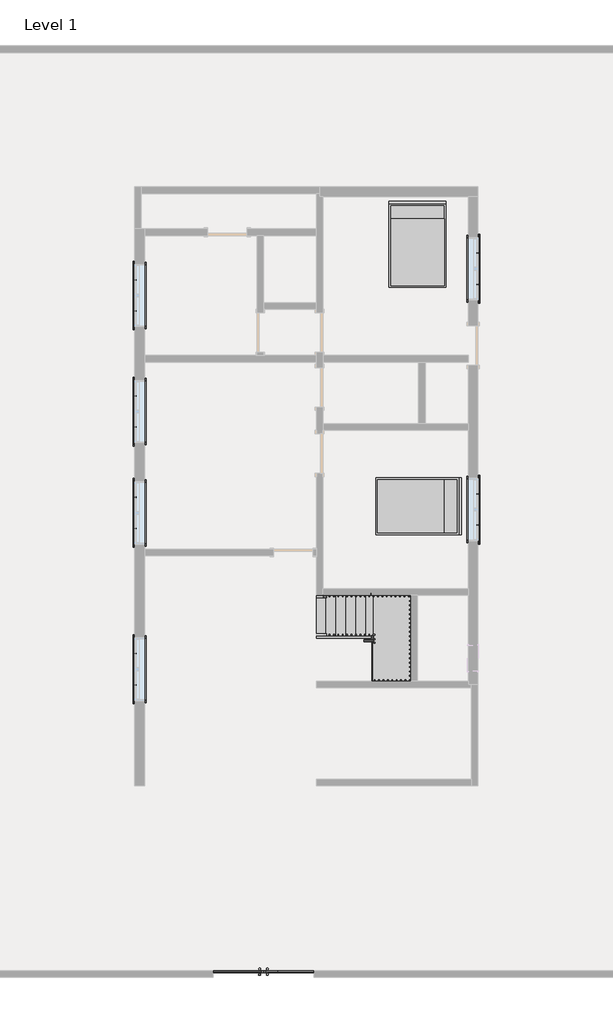
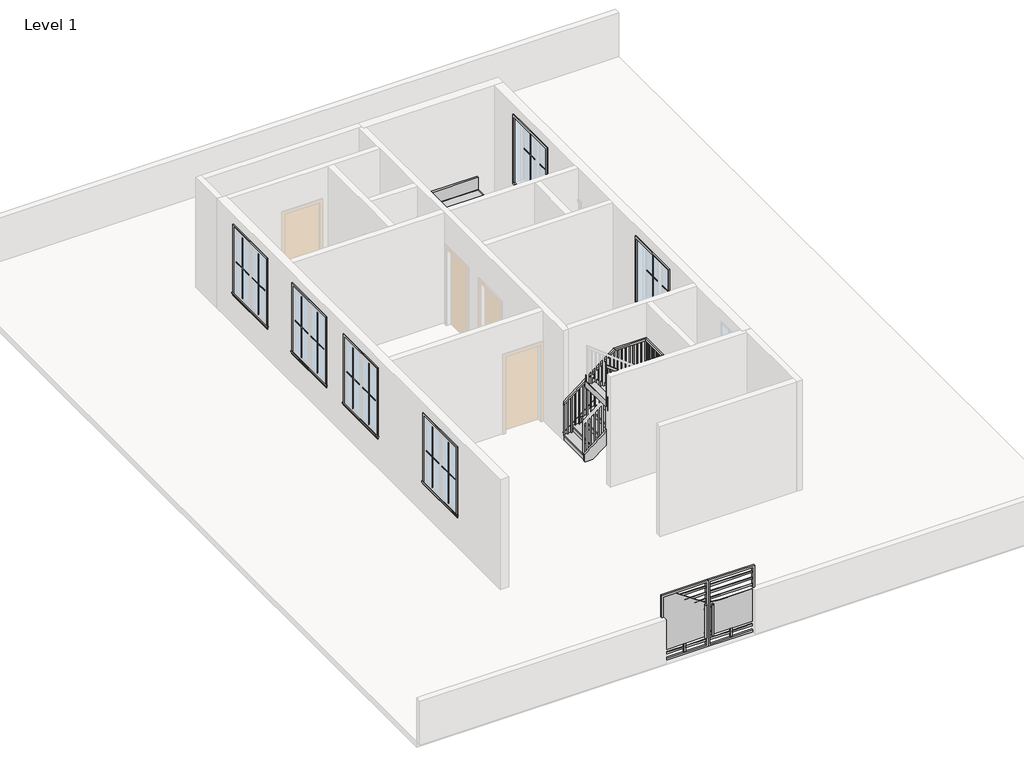
# One storey, part 2 of 2: 25 proxies, 6 members, 2 furniture elements, 1 railing, 1 stair flight.
"""IFC4 building model written with IfcOpenShell, lengths in millimetres."""

from ifc_helpers import new_model, si_unit, frame, origin, place, context, project, spatial, polyline, outline, extrude, faceted_brep, transform, mapped, element, save
from components import generic_models_113f6068, muntin_pattern_2x2_muntin_pattern_2x2_bff912c5, muntin_pattern_2x2_muntin_pattern_2x2_c2194282, trim_window_exterior_flat_with_sill_e04b3088, trim_window_interior_flat_picture_frame_2a7685fe, bed_17739_bed_17739_15c61121, stair_flight_3a0fea93

model = new_model("IFC4")

# Units and contexts
model_context = context("Model", 3, world=origin())
ifc_project = project(units=[si_unit("LENGTHUNIT", "METRE", prefix="MILLI")], contexts=[model_context])

# Site, building, storey
site = spatial("IfcSite", under=ifc_project)
building = spatial("IfcBuilding", under=site)
storey = spatial("IfcBuildingStorey", under=building, Name="Level 1", Elevation=0.0)

# Proxies
placement = place(None, origin())
generic_models_shape = generic_models_113f6068(model_context)
element("IfcBuildingElementProxy", 1, Name="Generic Models", at=placement, inside=storey, context=model_context, shape_type="MappedRepresentation", body=[
    mapped(generic_models_shape, transform((-2241.8415352, -11585.888028, 0.0), x_axis=(1.0, 0.0, 0.0), y_axis=(0.0, 1.0, 0.0), z_axis=(0.0, 0.0, 1.0))),
])
muntin_pattern_2x2_muntin_pattern_2x2_shape = muntin_pattern_2x2_muntin_pattern_2x2_bff912c5(model_context)
element("IfcBuildingElementProxy", 2, Name="Muntin Pattern_2x2 : Muntin Pattern_2x2", ObjectType="Muntin Pattern_2x2 : Muntin Pattern_2x2", at=placement, inside=storey, context=model_context, shape_type="MappedRepresentation", body=[
    mapped(muntin_pattern_2x2_muntin_pattern_2x2_shape, transform((-5204.1165352, 3633.8812696, 984.25), x_axis=(0.0, 1.0, 0.0), y_axis=(-1.0, 0.0, 0.0), z_axis=(0.0, 0.0, 1.0))),
])
element("IfcBuildingElementProxy", 3, Name="Muntin Pattern_2x2 : Muntin Pattern_2x2", ObjectType="Muntin Pattern_2x2 : Muntin Pattern_2x2", at=placement, inside=storey, context=model_context, shape_type="MappedRepresentation", body=[
    mapped(muntin_pattern_2x2_muntin_pattern_2x2_shape, transform((2701.6334648, 4971.3355313, 984.25), x_axis=(0.0, -1.0, 0.0), y_axis=(1.0, 0.0, 0.0), z_axis=(0.0, 0.0, 1.0))),
])
element("IfcBuildingElementProxy", 4, Name="Muntin Pattern_2x2 : Muntin Pattern_2x2", ObjectType="Muntin Pattern_2x2 : Muntin Pattern_2x2", at=placement, inside=storey, context=model_context, shape_type="MappedRepresentation", body=[
    mapped(muntin_pattern_2x2_muntin_pattern_2x2_shape, transform((2701.6334648, -584.9144687, 984.25), x_axis=(0.0, -1.0, 0.0), y_axis=(1.0, 0.0, 0.0), z_axis=(0.0, 0.0, 1.0))),
])
element("IfcBuildingElementProxy", 5, Name="Muntin Pattern_2x2 : Muntin Pattern_2x2", ObjectType="Muntin Pattern_2x2 : Muntin Pattern_2x2", at=placement, inside=storey, context=model_context, shape_type="MappedRepresentation", body=[
    mapped(muntin_pattern_2x2_muntin_pattern_2x2_shape, transform((-5204.1165352, 954.9605313, 984.25), x_axis=(0.0, 1.0, 0.0), y_axis=(-1.0, 0.0, 0.0), z_axis=(0.0, 0.0, 1.0))),
])
element("IfcBuildingElementProxy", 6, Name="Muntin Pattern_2x2 : Muntin Pattern_2x2", ObjectType="Muntin Pattern_2x2 : Muntin Pattern_2x2", at=placement, inside=storey, context=model_context, shape_type="MappedRepresentation", body=[
    mapped(muntin_pattern_2x2_muntin_pattern_2x2_shape, transform((-5204.1165352, -1381.8394687, 984.25), x_axis=(0.0, 1.0, 0.0), y_axis=(-1.0, 0.0, 0.0), z_axis=(0.0, 0.0, 1.0))),
])
element("IfcBuildingElementProxy", 7, Name="Muntin Pattern_2x2 : Muntin Pattern_2x2", ObjectType="Muntin Pattern_2x2 : Muntin Pattern_2x2", at=placement, inside=storey, context=model_context, shape_type="MappedRepresentation", body=[
    mapped(muntin_pattern_2x2_muntin_pattern_2x2_shape, transform((-5204.1165352, -4988.6394687, 984.25), x_axis=(0.0, 1.0, 0.0), y_axis=(-1.0, 0.0, 0.0), z_axis=(0.0, 0.0, 1.0))),
])
muntin_pattern_2x2_muntin_pattern_2x2_2_shape = muntin_pattern_2x2_muntin_pattern_2x2_c2194282(model_context)
element("IfcBuildingElementProxy", 8, Name="Muntin Pattern_2x2 : Muntin Pattern_2x2", ObjectType="Muntin Pattern_2x2 : Muntin Pattern_2x2", at=placement, inside=storey, context=model_context, shape_type="MappedRepresentation", body=[
    mapped(muntin_pattern_2x2_muntin_pattern_2x2_2_shape, transform((-5204.1165352, 4354.6062696, 984.25), x_axis=(0.0, -1.0, 0.0), y_axis=(1.0, 0.0, 0.0), z_axis=(0.0, 0.0, 1.0))),
])
element("IfcBuildingElementProxy", 9, Name="Muntin Pattern_2x2 : Muntin Pattern_2x2", ObjectType="Muntin Pattern_2x2 : Muntin Pattern_2x2", at=placement, inside=storey, context=model_context, shape_type="MappedRepresentation", body=[
    mapped(muntin_pattern_2x2_muntin_pattern_2x2_2_shape, transform((2701.6334648, 4250.6105313, 984.25), x_axis=(0.0, 1.0, 0.0), y_axis=(-1.0, 0.0, 0.0), z_axis=(0.0, 0.0, 1.0))),
])
element("IfcBuildingElementProxy", 10, Name="Muntin Pattern_2x2 : Muntin Pattern_2x2", ObjectType="Muntin Pattern_2x2 : Muntin Pattern_2x2", at=placement, inside=storey, context=model_context, shape_type="MappedRepresentation", body=[
    mapped(muntin_pattern_2x2_muntin_pattern_2x2_2_shape, transform((2701.6334648, -1305.6394687, 984.25), x_axis=(0.0, 1.0, 0.0), y_axis=(-1.0, 0.0, 0.0), z_axis=(0.0, 0.0, 1.0))),
])
element("IfcBuildingElementProxy", 11, Name="Muntin Pattern_2x2 : Muntin Pattern_2x2", ObjectType="Muntin Pattern_2x2 : Muntin Pattern_2x2", at=placement, inside=storey, context=model_context, shape_type="MappedRepresentation", body=[
    mapped(muntin_pattern_2x2_muntin_pattern_2x2_2_shape, transform((-5204.1165352, 1675.6855313, 984.25), x_axis=(0.0, -1.0, 0.0), y_axis=(1.0, 0.0, 0.0), z_axis=(0.0, 0.0, 1.0))),
])
element("IfcBuildingElementProxy", 12, Name="Muntin Pattern_2x2 : Muntin Pattern_2x2", ObjectType="Muntin Pattern_2x2 : Muntin Pattern_2x2", at=placement, inside=storey, context=model_context, shape_type="MappedRepresentation", body=[
    mapped(muntin_pattern_2x2_muntin_pattern_2x2_2_shape, transform((-5204.1165352, -661.1144687, 984.25), x_axis=(0.0, -1.0, 0.0), y_axis=(1.0, 0.0, 0.0), z_axis=(0.0, 0.0, 1.0))),
])
element("IfcBuildingElementProxy", 13, Name="Muntin Pattern_2x2 : Muntin Pattern_2x2", ObjectType="Muntin Pattern_2x2 : Muntin Pattern_2x2", at=placement, inside=storey, context=model_context, shape_type="MappedRepresentation", body=[
    mapped(muntin_pattern_2x2_muntin_pattern_2x2_2_shape, transform((-5204.1165352, -4267.9144687, 984.25), x_axis=(0.0, -1.0, 0.0), y_axis=(1.0, 0.0, 0.0), z_axis=(0.0, 0.0, 1.0))),
])
trim_window_exterior_flat_with_sill_shape = trim_window_exterior_flat_with_sill_e04b3088(model_context)
element("IfcBuildingElementProxy", 14, Name="Trim-Window-Exterior-Flat : with Sill", ObjectType="Trim-Window-Exterior-Flat : with Sill", at=placement, inside=storey, context=model_context, shape_type="MappedRepresentation", body=[
    mapped(trim_window_exterior_flat_with_sill_shape, transform((-5213.6415352, 3994.2437696, 2743.2), x_axis=(0.0, -1.0, 0.0), y_axis=(0.0, 0.0, 1.0), z_axis=(-1.0, 0.0, 0.0))),
])
element("IfcBuildingElementProxy", 15, Name="Trim-Window-Exterior-Flat : with Sill", ObjectType="Trim-Window-Exterior-Flat : with Sill", at=placement, inside=storey, context=model_context, shape_type="MappedRepresentation", body=[
    mapped(trim_window_exterior_flat_with_sill_shape, transform((2711.1584648, 4610.9730313, 2743.2), x_axis=(0.0, 1.0, 0.0), y_axis=(0.0, 0.0, 1.0), z_axis=(1.0, 0.0, 0.0))),
])
element("IfcBuildingElementProxy", 16, Name="Trim-Window-Exterior-Flat : with Sill", ObjectType="Trim-Window-Exterior-Flat : with Sill", at=placement, inside=storey, context=model_context, shape_type="MappedRepresentation", body=[
    mapped(trim_window_exterior_flat_with_sill_shape, transform((2711.1584648, -945.2769687, 2743.2), x_axis=(0.0, 1.0, 0.0), y_axis=(0.0, 0.0, 1.0), z_axis=(1.0, 0.0, 0.0))),
])
element("IfcBuildingElementProxy", 17, Name="Trim-Window-Exterior-Flat : with Sill", ObjectType="Trim-Window-Exterior-Flat : with Sill", at=placement, inside=storey, context=model_context, shape_type="MappedRepresentation", body=[
    mapped(trim_window_exterior_flat_with_sill_shape, transform((-5213.6415352, 1315.3230313, 2743.2), x_axis=(0.0, -1.0, 0.0), y_axis=(0.0, 0.0, 1.0), z_axis=(-1.0, 0.0, 0.0))),
])
element("IfcBuildingElementProxy", 18, Name="Trim-Window-Exterior-Flat : with Sill", ObjectType="Trim-Window-Exterior-Flat : with Sill", at=placement, inside=storey, context=model_context, shape_type="MappedRepresentation", body=[
    mapped(trim_window_exterior_flat_with_sill_shape, transform((-5213.6415352, -1021.4769687, 2743.2), x_axis=(0.0, -1.0, 0.0), y_axis=(0.0, 0.0, 1.0), z_axis=(-1.0, 0.0, 0.0))),
])
element("IfcBuildingElementProxy", 19, Name="Trim-Window-Exterior-Flat : with Sill", ObjectType="Trim-Window-Exterior-Flat : with Sill", at=placement, inside=storey, context=model_context, shape_type="MappedRepresentation", body=[
    mapped(trim_window_exterior_flat_with_sill_shape, transform((-5213.6415352, -4628.2769687, 2743.2), x_axis=(0.0, -1.0, 0.0), y_axis=(0.0, 0.0, 1.0), z_axis=(-1.0, 0.0, 0.0))),
])
trim_window_interior_flat_picture_frame_shape = trim_window_interior_flat_picture_frame_2a7685fe(model_context)
element("IfcBuildingElementProxy", 20, Name="Trim-Window-Interior-Flat : Picture Frame", ObjectType="Trim-Window-Interior-Flat : Picture Frame", at=placement, inside=storey, context=model_context, shape_type="MappedRepresentation", body=[
    mapped(trim_window_interior_flat_picture_frame_shape, transform((-4985.0415352, 3994.2437696, 2743.2), x_axis=(0.0, 1.0, 0.0), y_axis=(0.0, 0.0, 1.0), z_axis=(1.0, 0.0, 0.0))),
])
element("IfcBuildingElementProxy", 21, Name="Trim-Window-Interior-Flat : Picture Frame", ObjectType="Trim-Window-Interior-Flat : Picture Frame", at=placement, inside=storey, context=model_context, shape_type="MappedRepresentation", body=[
    mapped(trim_window_interior_flat_picture_frame_shape, transform((2482.5584648, 4610.9730313, 2743.2), x_axis=(0.0, -1.0, 0.0), y_axis=(0.0, 0.0, 1.0), z_axis=(-1.0, 0.0, 0.0))),
])
element("IfcBuildingElementProxy", 22, Name="Trim-Window-Interior-Flat : Picture Frame", ObjectType="Trim-Window-Interior-Flat : Picture Frame", at=placement, inside=storey, context=model_context, shape_type="MappedRepresentation", body=[
    mapped(trim_window_interior_flat_picture_frame_shape, transform((2482.5584648, -945.2769687, 2743.2), x_axis=(0.0, -1.0, 0.0), y_axis=(0.0, 0.0, 1.0), z_axis=(-1.0, 0.0, 0.0))),
])
element("IfcBuildingElementProxy", 23, Name="Trim-Window-Interior-Flat : Picture Frame", ObjectType="Trim-Window-Interior-Flat : Picture Frame", at=placement, inside=storey, context=model_context, shape_type="MappedRepresentation", body=[
    mapped(trim_window_interior_flat_picture_frame_shape, transform((-4985.0415352, 1315.3230313, 2743.2), x_axis=(0.0, 1.0, 0.0), y_axis=(0.0, 0.0, 1.0), z_axis=(1.0, 0.0, 0.0))),
])
element("IfcBuildingElementProxy", 24, Name="Trim-Window-Interior-Flat : Picture Frame", ObjectType="Trim-Window-Interior-Flat : Picture Frame", at=placement, inside=storey, context=model_context, shape_type="MappedRepresentation", body=[
    mapped(trim_window_interior_flat_picture_frame_shape, transform((-4985.0415352, -1021.4769687, 2743.2), x_axis=(0.0, 1.0, 0.0), y_axis=(0.0, 0.0, 1.0), z_axis=(1.0, 0.0, 0.0))),
])
element("IfcBuildingElementProxy", 25, Name="Trim-Window-Interior-Flat : Picture Frame", ObjectType="Trim-Window-Interior-Flat : Picture Frame", at=placement, inside=storey, context=model_context, shape_type="MappedRepresentation", body=[
    mapped(trim_window_interior_flat_picture_frame_shape, transform((-4985.0415352, -4628.2769687, 2743.2), x_axis=(0.0, 1.0, 0.0), y_axis=(0.0, 0.0, 1.0), z_axis=(1.0, 0.0, 0.0))),
])

# Furniture
bed_17739_bed_17739_shape = bed_17739_bed_17739_15c61121(model_context)
element("IfcFurniture", 26, ObjectType="Bed_17739 : Bed_17739", at=placement, inside=storey, context=model_context, shape_type="MappedRepresentation", body=[
    mapped(bed_17739_bed_17739_shape, transform((1314.1584648, 5149.1645078, 0.0), x_axis=(1.0, 0.0, 0.0), y_axis=(0.0, 1.0, 0.0), z_axis=(0.0, 0.0, 1.0))),
])
element("IfcFurniture", 27, ObjectType="Bed_17739 : Bed_17739", at=placement, inside=storey, context=model_context, shape_type="MappedRepresentation", body=[
    mapped(bed_17739_bed_17739_shape, transform((1314.1584648, -869.0769687, 0.0), x_axis=(0.0, -1.0, 0.0), y_axis=(1.0, 0.0, 0.0), z_axis=(0.0, 0.0, 1.0))),
])

# Members
element("IfcMember", 28, ObjectType="Stringer - 2\" Width", at=placement, inside=storey, context=model_context, shape_type="SweptSolid", body=[
    extrude(outline(polyline([(221.7399812, -1022.6415352), (0.0, -1022.6415352), (0.0, -811.2687863), (1261.5333333, 810.8400359), (1261.5333333, 314.3488758), (221.7399812, -1022.6415352)])), frame((0.0, -2926.4769687, 0.0), z_axis=(0.0, 1.0, 0.0), x_axis=(0.0, 0.0, 1.0)), (0.0, 0.0, 1.0), 50.8),
])
element("IfcMember", 29, ObjectType="Stringer - 2\" Width", at=placement, inside=storey, context=model_context, shape_type="SweptSolid", body=[
    extrude(outline(polyline([(1161.7584648, -2875.6769687), (1212.5584648, -2875.6769687), (1212.5584648, -4907.6769687), (1161.7584648, -4907.6769687), (1161.7584648, -2875.6769687)])), frame((0.0, 0.0, 956.7333333), z_axis=(0.0, 0.0, 1.0), x_axis=(1.0, 0.0, 0.0)), (0.0, 0.0, 1.0), 304.8),
])
element("IfcMember", 30, ObjectType="Stringer - 2\" Width", at=placement, inside=storey, context=model_context, shape_type="SweptSolid", body=[
    extrude(outline(polyline([(956.7333333, 884.5469698), (2439.9765283, -1022.6415352), (2053.8494451, -1022.6415352), (956.7333333, 388.0558097), (956.7333333, 884.5469698)])), frame((0.0, -4958.4769687, 0.0), z_axis=(0.0, 1.0, 0.0), x_axis=(0.0, 0.0, 1.0)), (0.0, 0.0, 1.0), 50.8),
])
element("IfcMember", 31, ObjectType="Stringer - 2\" Width", at=placement, inside=storey, context=model_context, shape_type="SweptSolid", body=[
    extrude(outline(polyline([(221.7399812, -1022.6415352), (0.0, -1022.6415352), (0.0, -811.2687863), (820.5567404, 243.8221038), (1206.6838236, 243.8221038), (221.7399812, -1022.6415352)])), frame((0.0, -3912.0539367, 0.0), z_axis=(0.0, 1.0, 0.0), x_axis=(0.0, 0.0, 1.0)), (0.0, 0.0, 1.0), 50.8),
])
element("IfcMember", 32, ObjectType="Stringer - 2\" Width", at=placement, inside=storey, context=model_context, shape_type="SweptSolid", body=[
    extrude(outline(polyline([(243.8221038, -3861.2539367), (294.6221038, -3861.2539367), (294.6221038, -3942.4769687), (243.8221038, -3942.4769687), (243.8221038, -3861.2539367)])), frame((0.0, 0.0, 956.7333333), z_axis=(0.0, 0.0, 1.0), x_axis=(1.0, 0.0, 0.0)), (0.0, 0.0, 1.0), 304.8),
])
element("IfcMember", 33, ObjectType="Stringer - 2\" Width", at=placement, inside=storey, context=model_context, shape_type="SweptSolid", body=[
    extrude(outline(polyline([(1029.3978382, 294.6221038), (1415.5249214, 294.6221038), (2439.9765283, -1022.6415352), (2053.8494451, -1022.6415352), (1029.3978382, 294.6221038)])), frame((0.0, -3993.2769687, 0.0), z_axis=(0.0, 1.0, 0.0), x_axis=(0.0, 0.0, 1.0)), (0.0, 0.0, 1.0), 50.8),
])

# Railing
element("IfcRailing", 34, ObjectType="Handrail - Rectangular", at=placement, inside=storey, context=model_context, shape_type="SolidModel", body=[
    faceted_brep([(-1022.6415352, -2926.4769687, 1083.7333333), (-1022.6415352, -2926.4769687, 1019.5783974), (-1022.6415352, -2977.2769687, 1019.5783974), (-1022.6415352, -2977.2769687, 1083.7333333), (294.6221038, -2926.4769687, 2099.7333333), (311.9370364, -2926.4769687, 2048.9333333), (311.9370364, -2977.2769687, 2048.9333333), (294.6221038, -2977.2769687, 2099.7333333), (1161.7584648, -2926.4769687, 2099.7333333), (1161.7584648, -2926.4769687, 2048.9333333), (1110.9584648, -2977.2769687, 2048.9333333), (1110.9584648, -2977.2769687, 2099.7333333), (1161.7584648, -4907.6769687, 2099.7333333), (1161.7584648, -4907.6769687, 2048.9333333), (1110.9584648, -4856.8769687, 2048.9333333), (1110.9584648, -4856.8769687, 2099.7333333), (514.1660437, -4907.6769687, 2099.7333333), (496.8511111, -4907.6769687, 2048.9333333), (496.8511111, -4856.8769687, 2048.9333333), (514.1660437, -4856.8769687, 2099.7333333), (-1022.6415352, -4907.6769687, 3285.0666667), (-1022.6415352, -4856.8769687, 3285.0666667), (-1022.6415352, -4856.8769687, 3220.9117307), (-1022.6415352, -4907.6769687, 3220.9117307)], [[[0, 1, 2, 3]], [[1, 0, 4, 5]], [[2, 1, 5, 6]], [[3, 2, 6, 7]], [[0, 3, 7, 4]], [[5, 4, 8, 9]], [[6, 5, 9, 10]], [[7, 6, 10, 11]], [[4, 7, 11, 8]], [[9, 8, 12, 13]], [[10, 9, 13, 14]], [[11, 10, 14, 15]], [[8, 11, 15, 12]], [[13, 12, 16, 17]], [[14, 13, 17, 18]], [[15, 14, 18, 19]], [[12, 15, 19, 16]], [[20, 21, 22, 23]], [[17, 16, 20, 23]], [[18, 17, 23, 22]], [[19, 18, 22, 21]], [[16, 19, 21, 20]]]),
    extrude(outline(polyline([(3208.6674089, -1006.7665352), (2201.3333333, -1006.7665352), (2201.3333333, -987.7165352), (3193.9742226, -987.7165352), (3208.6674089, -1006.7665352)])), frame((0.0, -4891.8019687, 0.0), z_axis=(0.0, 1.0, 0.0), x_axis=(0.0, 0.0, 1.0)), (0.0, 0.0, 1.0), 19.05),
    extrude(outline(polyline([(3130.3037488, -905.1665352), (2201.3333333, -905.1665352), (2201.3333333, -886.1165352), (3115.6105626, -886.1165352), (3130.3037488, -905.1665352)])), frame((0.0, -4891.8019687, 0.0), z_axis=(0.0, 1.0, 0.0), x_axis=(0.0, 0.0, 1.0)), (0.0, 0.0, 1.0), 19.05),
    extrude(outline(polyline([(3051.9400888, -803.5665352), (2201.3333333, -803.5665352), (2201.3333333, -784.5165352), (3037.2469025, -784.5165352), (3051.9400888, -803.5665352)])), frame((0.0, -4891.8019687, 0.0), z_axis=(0.0, 1.0, 0.0), x_axis=(0.0, 0.0, 1.0)), (0.0, 0.0, 1.0), 19.05),
    extrude(outline(polyline([(2973.5764287, -701.9665352), (2032.0, -701.9665352), (2032.0, -682.9165352), (2958.8832425, -682.9165352), (2973.5764287, -701.9665352)])), frame((0.0, -4891.8019687, 0.0), z_axis=(0.0, 1.0, 0.0), x_axis=(0.0, 0.0, 1.0)), (0.0, 0.0, 1.0), 19.05),
    extrude(outline(polyline([(2895.2127687, -600.3665352), (2032.0, -600.3665352), (2032.0, -581.3165352), (2880.5195824, -581.3165352), (2895.2127687, -600.3665352)])), frame((0.0, -4891.8019687, 0.0), z_axis=(0.0, 1.0, 0.0), x_axis=(0.0, 0.0, 1.0)), (0.0, 0.0, 1.0), 19.05),
    extrude(outline(polyline([(2816.8491086, -498.7665352), (1862.6666667, -498.7665352), (1862.6666667, -479.7165352), (2802.1559224, -479.7165352), (2816.8491086, -498.7665352)])), frame((0.0, -4891.8019687, 0.0), z_axis=(0.0, 1.0, 0.0), x_axis=(0.0, 0.0, 1.0)), (0.0, 0.0, 1.0), 19.05),
    extrude(outline(polyline([(2738.4854486, -397.1665352), (1862.6666667, -397.1665352), (1862.6666667, -378.1165352), (2723.7922623, -378.1165352), (2738.4854486, -397.1665352)])), frame((0.0, -4891.8019687, 0.0), z_axis=(0.0, 1.0, 0.0), x_axis=(0.0, 0.0, 1.0)), (0.0, 0.0, 1.0), 19.05),
    extrude(outline(polyline([(2660.1217885, -295.5665352), (1693.3333333, -295.5665352), (1693.3333333, -276.5165352), (2645.4286023, -276.5165352), (2660.1217885, -295.5665352)])), frame((0.0, -4891.8019687, 0.0), z_axis=(0.0, 1.0, 0.0), x_axis=(0.0, 0.0, 1.0)), (0.0, 0.0, 1.0), 19.05),
    extrude(outline(polyline([(2581.7581285, -193.9665352), (1693.3333333, -193.9665352), (1693.3333333, -174.9165352), (2567.0649422, -174.9165352), (2581.7581285, -193.9665352)])), frame((0.0, -4891.8019687, 0.0), z_axis=(0.0, 1.0, 0.0), x_axis=(0.0, 0.0, 1.0)), (0.0, 0.0, 1.0), 19.05),
    extrude(outline(polyline([(2503.3944684, -92.3665352), (1524.0, -92.3665352), (1524.0, -73.3165352), (2488.7012822, -73.3165352), (2503.3944684, -92.3665352)])), frame((0.0, -4891.8019687, 0.0), z_axis=(0.0, 1.0, 0.0), x_axis=(0.0, 0.0, 1.0)), (0.0, 0.0, 1.0), 19.05),
    extrude(outline(polyline([(2425.0308084, 9.2334648), (1524.0, 9.2334648), (1524.0, 28.2834648), (2410.3376221, 28.2834648), (2425.0308084, 9.2334648)])), frame((0.0, -4891.8019687, 0.0), z_axis=(0.0, 1.0, 0.0), x_axis=(0.0, 0.0, 1.0)), (0.0, 0.0, 1.0), 19.05),
    extrude(outline(polyline([(2346.6671484, 110.8334648), (1524.0, 110.8334648), (1524.0, 129.8834648), (2331.9739621, 129.8834648), (2346.6671484, 110.8334648)])), frame((0.0, -4891.8019687, 0.0), z_axis=(0.0, 1.0, 0.0), x_axis=(0.0, 0.0, 1.0)), (0.0, 0.0, 1.0), 19.05),
    extrude(outline(polyline([(2268.3034883, 212.4334648), (1354.6666667, 212.4334648), (1354.6666667, 231.4834648), (2253.6103021, 231.4834648), (2268.3034883, 212.4334648)])), frame((0.0, -4891.8019687, 0.0), z_axis=(0.0, 1.0, 0.0), x_axis=(0.0, 0.0, 1.0)), (0.0, 0.0, 1.0), 19.05),
    extrude(outline(polyline([(2189.9398283, 314.0334648), (1185.3333333, 314.0334648), (1185.3333333, 333.0834648), (2175.246642, 333.0834648), (2189.9398283, 314.0334648)])), frame((0.0, -4891.8019687, 0.0), z_axis=(0.0, 1.0, 0.0), x_axis=(0.0, 0.0, 1.0)), (0.0, 0.0, 1.0), 19.05),
    extrude(outline(polyline([(2111.5761682, 415.6334648), (1185.3333333, 415.6334648), (1185.3333333, 434.6834648), (2096.882982, 434.6834648), (2111.5761682, 415.6334648)])), frame((0.0, -4891.8019687, 0.0), z_axis=(0.0, 1.0, 0.0), x_axis=(0.0, 0.0, 1.0)), (0.0, 0.0, 1.0), 19.05),
    extrude(outline(polyline([(536.2834648, -4891.8019687), (517.2334648, -4891.8019687), (517.2334648, -4872.7519687), (536.2834648, -4872.7519687), (536.2834648, -4891.8019687)])), frame((0.0, 0.0, 1185.3333333), z_axis=(0.0, 0.0, 1.0), x_axis=(1.0, 0.0, 0.0)), (0.0, 0.0, 1.0), 863.6),
    extrude(outline(polyline([(637.8834648, -4891.8019687), (618.8334648, -4891.8019687), (618.8334648, -4872.7519687), (637.8834648, -4872.7519687), (637.8834648, -4891.8019687)])), frame((0.0, 0.0, 1185.3333333), z_axis=(0.0, 0.0, 1.0), x_axis=(1.0, 0.0, 0.0)), (0.0, 0.0, 1.0), 863.6),
    extrude(outline(polyline([(739.4834648, -4891.8019687), (720.4334648, -4891.8019687), (720.4334648, -4872.7519687), (739.4834648, -4872.7519687), (739.4834648, -4891.8019687)])), frame((0.0, 0.0, 1185.3333333), z_axis=(0.0, 0.0, 1.0), x_axis=(1.0, 0.0, 0.0)), (0.0, 0.0, 1.0), 863.6),
    extrude(outline(polyline([(841.0834648, -4891.8019687), (822.0334648, -4891.8019687), (822.0334648, -4872.7519687), (841.0834648, -4872.7519687), (841.0834648, -4891.8019687)])), frame((0.0, 0.0, 1185.3333333), z_axis=(0.0, 0.0, 1.0), x_axis=(1.0, 0.0, 0.0)), (0.0, 0.0, 1.0), 863.6),
    extrude(outline(polyline([(942.6834648, -4891.8019687), (923.6334648, -4891.8019687), (923.6334648, -4872.7519687), (942.6834648, -4872.7519687), (942.6834648, -4891.8019687)])), frame((0.0, 0.0, 1185.3333333), z_axis=(0.0, 0.0, 1.0), x_axis=(1.0, 0.0, 0.0)), (0.0, 0.0, 1.0), 863.6),
    extrude(outline(polyline([(1044.2834648, -4891.8019687), (1025.2334648, -4891.8019687), (1025.2334648, -4872.7519687), (1044.2834648, -4872.7519687), (1044.2834648, -4891.8019687)])), frame((0.0, 0.0, 1185.3333333), z_axis=(0.0, 0.0, 1.0), x_axis=(1.0, 0.0, 0.0)), (0.0, 0.0, 1.0), 863.6),
    extrude(outline(polyline([(1145.8834648, -4771.1519687), (1145.8834648, -4790.2019687), (1126.8334648, -4790.2019687), (1126.8334648, -4771.1519687), (1145.8834648, -4771.1519687)])), frame((0.0, 0.0, 1185.3333333), z_axis=(0.0, 0.0, 1.0), x_axis=(1.0, 0.0, 0.0)), (0.0, 0.0, 1.0), 863.6),
    extrude(outline(polyline([(1145.8834648, -4669.5519687), (1145.8834648, -4688.6019687), (1126.8334648, -4688.6019687), (1126.8334648, -4669.5519687), (1145.8834648, -4669.5519687)])), frame((0.0, 0.0, 1185.3333333), z_axis=(0.0, 0.0, 1.0), x_axis=(1.0, 0.0, 0.0)), (0.0, 0.0, 1.0), 863.6),
    extrude(outline(polyline([(1145.8834648, -4567.9519687), (1145.8834648, -4587.0019687), (1126.8334648, -4587.0019687), (1126.8334648, -4567.9519687), (1145.8834648, -4567.9519687)])), frame((0.0, 0.0, 1185.3333333), z_axis=(0.0, 0.0, 1.0), x_axis=(1.0, 0.0, 0.0)), (0.0, 0.0, 1.0), 863.6),
    extrude(outline(polyline([(1145.8834648, -4466.3519687), (1145.8834648, -4485.4019687), (1126.8334648, -4485.4019687), (1126.8334648, -4466.3519687), (1145.8834648, -4466.3519687)])), frame((0.0, 0.0, 1185.3333333), z_axis=(0.0, 0.0, 1.0), x_axis=(1.0, 0.0, 0.0)), (0.0, 0.0, 1.0), 863.6),
    extrude(outline(polyline([(1145.8834648, -4364.7519687), (1145.8834648, -4383.8019687), (1126.8334648, -4383.8019687), (1126.8334648, -4364.7519687), (1145.8834648, -4364.7519687)])), frame((0.0, 0.0, 1185.3333333), z_axis=(0.0, 0.0, 1.0), x_axis=(1.0, 0.0, 0.0)), (0.0, 0.0, 1.0), 863.6),
    extrude(outline(polyline([(1145.8834648, -4263.1519687), (1145.8834648, -4282.2019687), (1126.8334648, -4282.2019687), (1126.8334648, -4263.1519687), (1145.8834648, -4263.1519687)])), frame((0.0, 0.0, 1185.3333333), z_axis=(0.0, 0.0, 1.0), x_axis=(1.0, 0.0, 0.0)), (0.0, 0.0, 1.0), 863.6),
    extrude(outline(polyline([(1145.8834648, -4161.5519687), (1145.8834648, -4180.6019687), (1126.8334648, -4180.6019687), (1126.8334648, -4161.5519687), (1145.8834648, -4161.5519687)])), frame((0.0, 0.0, 1185.3333333), z_axis=(0.0, 0.0, 1.0), x_axis=(1.0, 0.0, 0.0)), (0.0, 0.0, 1.0), 863.6),
    extrude(outline(polyline([(1145.8834648, -4059.9519687), (1145.8834648, -4079.0019687), (1126.8334648, -4079.0019687), (1126.8334648, -4059.9519687), (1145.8834648, -4059.9519687)])), frame((0.0, 0.0, 1185.3333333), z_axis=(0.0, 0.0, 1.0), x_axis=(1.0, 0.0, 0.0)), (0.0, 0.0, 1.0), 863.6),
    extrude(outline(polyline([(1145.8834648, -3958.3519687), (1145.8834648, -3977.4019687), (1126.8334648, -3977.4019687), (1126.8334648, -3958.3519687), (1145.8834648, -3958.3519687)])), frame((0.0, 0.0, 1185.3333333), z_axis=(0.0, 0.0, 1.0), x_axis=(1.0, 0.0, 0.0)), (0.0, 0.0, 1.0), 863.6),
    extrude(outline(polyline([(1145.8834648, -3856.7519687), (1145.8834648, -3875.8019687), (1126.8334648, -3875.8019687), (1126.8334648, -3856.7519687), (1145.8834648, -3856.7519687)])), frame((0.0, 0.0, 1185.3333333), z_axis=(0.0, 0.0, 1.0), x_axis=(1.0, 0.0, 0.0)), (0.0, 0.0, 1.0), 863.6),
    extrude(outline(polyline([(1145.8834648, -3755.1519687), (1145.8834648, -3774.2019687), (1126.8334648, -3774.2019687), (1126.8334648, -3755.1519687), (1145.8834648, -3755.1519687)])), frame((0.0, 0.0, 1185.3333333), z_axis=(0.0, 0.0, 1.0), x_axis=(1.0, 0.0, 0.0)), (0.0, 0.0, 1.0), 863.6),
    extrude(outline(polyline([(1145.8834648, -3653.5519687), (1145.8834648, -3672.6019687), (1126.8334648, -3672.6019687), (1126.8334648, -3653.5519687), (1145.8834648, -3653.5519687)])), frame((0.0, 0.0, 1185.3333333), z_axis=(0.0, 0.0, 1.0), x_axis=(1.0, 0.0, 0.0)), (0.0, 0.0, 1.0), 863.6),
    extrude(outline(polyline([(1145.8834648, -3551.9519687), (1145.8834648, -3571.0019687), (1126.8334648, -3571.0019687), (1126.8334648, -3551.9519687), (1145.8834648, -3551.9519687)])), frame((0.0, 0.0, 1185.3333333), z_axis=(0.0, 0.0, 1.0), x_axis=(1.0, 0.0, 0.0)), (0.0, 0.0, 1.0), 863.6),
    extrude(outline(polyline([(1145.8834648, -3450.3519687), (1145.8834648, -3469.4019687), (1126.8334648, -3469.4019687), (1126.8334648, -3450.3519687), (1145.8834648, -3450.3519687)])), frame((0.0, 0.0, 1185.3333333), z_axis=(0.0, 0.0, 1.0), x_axis=(1.0, 0.0, 0.0)), (0.0, 0.0, 1.0), 863.6),
    extrude(outline(polyline([(1145.8834648, -3348.7519687), (1145.8834648, -3367.8019687), (1126.8334648, -3367.8019687), (1126.8334648, -3348.7519687), (1145.8834648, -3348.7519687)])), frame((0.0, 0.0, 1185.3333333), z_axis=(0.0, 0.0, 1.0), x_axis=(1.0, 0.0, 0.0)), (0.0, 0.0, 1.0), 863.6),
    extrude(outline(polyline([(1145.8834648, -3247.1519687), (1145.8834648, -3266.2019687), (1126.8334648, -3266.2019687), (1126.8334648, -3247.1519687), (1145.8834648, -3247.1519687)])), frame((0.0, 0.0, 1185.3333333), z_axis=(0.0, 0.0, 1.0), x_axis=(1.0, 0.0, 0.0)), (0.0, 0.0, 1.0), 863.6),
    extrude(outline(polyline([(1145.8834648, -3145.5519687), (1145.8834648, -3164.6019687), (1126.8334648, -3164.6019687), (1126.8334648, -3145.5519687), (1145.8834648, -3145.5519687)])), frame((0.0, 0.0, 1185.3333333), z_axis=(0.0, 0.0, 1.0), x_axis=(1.0, 0.0, 0.0)), (0.0, 0.0, 1.0), 863.6),
    extrude(outline(polyline([(1145.8834648, -3043.9519687), (1145.8834648, -3063.0019687), (1126.8334648, -3063.0019687), (1126.8334648, -3043.9519687), (1145.8834648, -3043.9519687)])), frame((0.0, 0.0, 1185.3333333), z_axis=(0.0, 0.0, 1.0), x_axis=(1.0, 0.0, 0.0)), (0.0, 0.0, 1.0), 863.6),
    extrude(outline(polyline([(1101.4334648, -2942.3519687), (1120.4834648, -2942.3519687), (1120.4834648, -2961.4019687), (1101.4334648, -2961.4019687), (1101.4334648, -2942.3519687)])), frame((0.0, 0.0, 1185.3333333), z_axis=(0.0, 0.0, 1.0), x_axis=(1.0, 0.0, 0.0)), (0.0, 0.0, 1.0), 863.6),
    extrude(outline(polyline([(999.8334648, -2942.3519687), (1018.8834648, -2942.3519687), (1018.8834648, -2961.4019687), (999.8334648, -2961.4019687), (999.8334648, -2942.3519687)])), frame((0.0, 0.0, 1185.3333333), z_axis=(0.0, 0.0, 1.0), x_axis=(1.0, 0.0, 0.0)), (0.0, 0.0, 1.0), 863.6),
    extrude(outline(polyline([(898.2334648, -2942.3519687), (917.2834648, -2942.3519687), (917.2834648, -2961.4019687), (898.2334648, -2961.4019687), (898.2334648, -2942.3519687)])), frame((0.0, 0.0, 1185.3333333), z_axis=(0.0, 0.0, 1.0), x_axis=(1.0, 0.0, 0.0)), (0.0, 0.0, 1.0), 863.6),
    extrude(outline(polyline([(796.6334648, -2942.3519687), (815.6834648, -2942.3519687), (815.6834648, -2961.4019687), (796.6334648, -2961.4019687), (796.6334648, -2942.3519687)])), frame((0.0, 0.0, 1185.3333333), z_axis=(0.0, 0.0, 1.0), x_axis=(1.0, 0.0, 0.0)), (0.0, 0.0, 1.0), 863.6),
    extrude(outline(polyline([(695.0334648, -2942.3519687), (714.0834648, -2942.3519687), (714.0834648, -2961.4019687), (695.0334648, -2961.4019687), (695.0334648, -2942.3519687)])), frame((0.0, 0.0, 1185.3333333), z_axis=(0.0, 0.0, 1.0), x_axis=(1.0, 0.0, 0.0)), (0.0, 0.0, 1.0), 863.6),
    extrude(outline(polyline([(593.4334648, -2942.3519687), (612.4834648, -2942.3519687), (612.4834648, -2961.4019687), (593.4334648, -2961.4019687), (593.4334648, -2942.3519687)])), frame((0.0, 0.0, 1185.3333333), z_axis=(0.0, 0.0, 1.0), x_axis=(1.0, 0.0, 0.0)), (0.0, 0.0, 1.0), 863.6),
    extrude(outline(polyline([(491.8334648, -2942.3519687), (510.8834648, -2942.3519687), (510.8834648, -2961.4019687), (491.8334648, -2961.4019687), (491.8334648, -2942.3519687)])), frame((0.0, 0.0, 1185.3333333), z_axis=(0.0, 0.0, 1.0), x_axis=(1.0, 0.0, 0.0)), (0.0, 0.0, 1.0), 863.6),
    extrude(outline(polyline([(390.2334648, -2942.3519687), (409.2834648, -2942.3519687), (409.2834648, -2961.4019687), (390.2334648, -2961.4019687), (390.2334648, -2942.3519687)])), frame((0.0, 0.0, 1185.3333333), z_axis=(0.0, 0.0, 1.0), x_axis=(1.0, 0.0, 0.0)), (0.0, 0.0, 1.0), 863.6),
    extrude(outline(polyline([(288.6334648, -2942.3519687), (307.6834648, -2942.3519687), (307.6834648, -2961.4019687), (288.6334648, -2961.4019687), (288.6334648, -2942.3519687)])), frame((0.0, 0.0, 1185.3333333), z_axis=(0.0, 0.0, 1.0), x_axis=(1.0, 0.0, 0.0)), (0.0, 0.0, 1.0), 863.6),
    extrude(outline(polyline([(1952.5957248, 187.0334648), (1016.0, 187.0334648), (1016.0, 206.0834648), (1967.2889111, 206.0834648), (1952.5957248, 187.0334648)])), frame((0.0, -2961.4019687, 0.0), z_axis=(0.0, 1.0, 0.0), x_axis=(0.0, 0.0, 1.0)), (0.0, 0.0, 1.0), 19.05),
    extrude(outline(polyline([(1874.2320648, 85.4334648), (846.6666667, 85.4334648), (846.6666667, 104.4834648), (1888.925251, 104.4834648), (1874.2320648, 85.4334648)])), frame((0.0, -2961.4019687, 0.0), z_axis=(0.0, 1.0, 0.0), x_axis=(0.0, 0.0, 1.0)), (0.0, 0.0, 1.0), 19.05),
    extrude(outline(polyline([(1795.8684047, -16.1665352), (846.6666667, -16.1665352), (846.6666667, 2.8834648), (1810.561591, 2.8834648), (1795.8684047, -16.1665352)])), frame((0.0, -2961.4019687, 0.0), z_axis=(0.0, 1.0, 0.0), x_axis=(0.0, 0.0, 1.0)), (0.0, 0.0, 1.0), 19.05),
    extrude(outline(polyline([(1717.5047447, -117.7665352), (846.6666667, -117.7665352), (846.6666667, -98.7165352), (1732.1979309, -98.7165352), (1717.5047447, -117.7665352)])), frame((0.0, -2961.4019687, 0.0), z_axis=(0.0, 1.0, 0.0), x_axis=(0.0, 0.0, 1.0)), (0.0, 0.0, 1.0), 19.05),
    extrude(outline(polyline([(1639.1410846, -219.3665352), (677.3333333, -219.3665352), (677.3333333, -200.3165352), (1653.8342709, -200.3165352), (1639.1410846, -219.3665352)])), frame((0.0, -2961.4019687, 0.0), z_axis=(0.0, 1.0, 0.0), x_axis=(0.0, 0.0, 1.0)), (0.0, 0.0, 1.0), 19.05),
    extrude(outline(polyline([(1560.7774246, -320.9665352), (677.3333333, -320.9665352), (677.3333333, -301.9165352), (1575.4706109, -301.9165352), (1560.7774246, -320.9665352)])), frame((0.0, -2961.4019687, 0.0), z_axis=(0.0, 1.0, 0.0), x_axis=(0.0, 0.0, 1.0)), (0.0, 0.0, 1.0), 19.05),
    extrude(outline(polyline([(1482.4137645, -422.5665352), (508.0, -422.5665352), (508.0, -403.5165352), (1497.1069508, -403.5165352), (1482.4137645, -422.5665352)])), frame((0.0, -2961.4019687, 0.0), z_axis=(0.0, 1.0, 0.0), x_axis=(0.0, 0.0, 1.0)), (0.0, 0.0, 1.0), 19.05),
    extrude(outline(polyline([(1404.0501045, -524.1665352), (508.0, -524.1665352), (508.0, -505.1165352), (1418.7432908, -505.1165352), (1404.0501045, -524.1665352)])), frame((0.0, -2961.4019687, 0.0), z_axis=(0.0, 1.0, 0.0), x_axis=(0.0, 0.0, 1.0)), (0.0, 0.0, 1.0), 19.05),
    extrude(outline(polyline([(1325.6864445, -625.7665352), (338.6666667, -625.7665352), (338.6666667, -606.7165352), (1340.3796307, -606.7165352), (1325.6864445, -625.7665352)])), frame((0.0, -2961.4019687, 0.0), z_axis=(0.0, 1.0, 0.0), x_axis=(0.0, 0.0, 1.0)), (0.0, 0.0, 1.0), 19.05),
    extrude(outline(polyline([(1247.3227844, -727.3665352), (338.6666667, -727.3665352), (338.6666667, -708.3165352), (1262.0159707, -708.3165352), (1247.3227844, -727.3665352)])), frame((0.0, -2961.4019687, 0.0), z_axis=(0.0, 1.0, 0.0), x_axis=(0.0, 0.0, 1.0)), (0.0, 0.0, 1.0), 19.05),
    extrude(outline(polyline([(1168.9591244, -828.9665352), (169.3333333, -828.9665352), (169.3333333, -809.9165352), (1183.6523106, -809.9165352), (1168.9591244, -828.9665352)])), frame((0.0, -2961.4019687, 0.0), z_axis=(0.0, 1.0, 0.0), x_axis=(0.0, 0.0, 1.0)), (0.0, 0.0, 1.0), 19.05),
    extrude(outline(polyline([(1090.5954643, -930.5665352), (169.3333333, -930.5665352), (169.3333333, -911.5165352), (1105.2886506, -911.5165352), (1090.5954643, -930.5665352)])), frame((0.0, -2961.4019687, 0.0), z_axis=(0.0, 1.0, 0.0), x_axis=(0.0, 0.0, 1.0)), (0.0, 0.0, 1.0), 19.05),
    extrude(outline(polyline([(1145.8834648, -4872.7519687), (1145.8834648, -4891.8019687), (1126.8334648, -4891.8019687), (1126.8334648, -4872.7519687), (1145.8834648, -4872.7519687)])), frame((0.0, 0.0, 1185.3333333), z_axis=(0.0, 0.0, 1.0), x_axis=(1.0, 0.0, 0.0)), (0.0, 0.0, 1.0), 863.6),
    extrude(outline(polyline([(1126.8334648, -2942.3519687), (1145.8834648, -2942.3519687), (1145.8834648, -2961.4019687), (1126.8334648, -2961.4019687), (1126.8334648, -2942.3519687)])), frame((0.0, 0.0, 1185.3333333), z_axis=(0.0, 0.0, 1.0), x_axis=(1.0, 0.0, 0.0)), (0.0, 0.0, 1.0), 863.6),
    extrude(outline(polyline([(3220.9117307, -1022.6415352), (2201.3333333, -1022.6415352), (2201.3333333, -1003.5915352), (3206.2185445, -1003.5915352), (3220.9117307, -1022.6415352)])), frame((0.0, -4891.8019687, 0.0), z_axis=(0.0, 1.0, 0.0), x_axis=(0.0, 0.0, 1.0)), (0.0, 0.0, 1.0), 19.05),
    extrude(outline(polyline([(1019.5783974, -1022.6415352), (169.3333333, -1022.6415352), (169.3333333, -1003.5915352), (1034.2715837, -1003.5915352), (1019.5783974, -1022.6415352)])), frame((0.0, -2961.4019687, 0.0), z_axis=(0.0, 1.0, 0.0), x_axis=(0.0, 0.0, 1.0)), (0.0, 0.0, 1.0), 19.05),
])

# Stair flight
stair_flight_shape = stair_flight_3a0fea93(model_context)
element("IfcStairFlight", 35, ObjectType="2\" Tread 1\" Nosing 1/4\" Riser", at=placement, inside=storey, context=model_context, shape_type="MappedRepresentation", body=[
    mapped(stair_flight_shape, transform((0.0, 0.0, 0.0), x_axis=(1.0, 0.0, 0.0), y_axis=(0.0, 1.0, 0.0), z_axis=(0.0, 0.0, 1.0))),
])

save(model, "model.ifc")

# Revit data of these elements
# Type
#   sheet = none
#   pipe = none
#   handal = none
#   faram = none
#   Default Elevation = 0
# Type "Muntin Pattern_2x2 : Muntin Pattern_2x2"
#   Width [instance default] = 4' - 0"
#   Thickness = 0' - 0 1/2"
#   Height [instance default] = 4' - 0"
#   Distance = 0' - 0 3/4"
#   Interior Material [instance default] = none
#   Exterior Material [instance default] = none
#   Default Elevation = 0
# Type "Trim-Window-Exterior-Flat : with Sill"
#   Trim Width = 0' - 2 1/4"
#   Trim Thickness_Picture Frame = 0' - 1 1/4"
#   Trim Thickness_with Sill = 0' - 0 3/4"
#   Sill Thickness = 0' - 1 1/4"
#   Opening Width [instance default] = 2' - 0"
#   Opening Height [instance default] = 3' - 0"
#   Default Elevation = 4' - 0"
#   Sill = yes
#   Picture Frame = no
#   Trim Material [instance default] = none
# Type "Trim-Window-Interior-Flat : Picture Frame"
#   Trim Thickness_Picture Frame = 0' - 1 1/4"
#   Trim Width = 0' - 2 1/4"
#   Trim Thickness_with Sill = 0' - 0 3/4"
#   Sill Thickness = 0' - 1 1/4"
#   Opening Width [instance default] = 2' - 0"
#   Opening Height [instance default] = 3' - 0"
#   Default Elevation = 4' - 0"
#   Sill = no
#   Picture Frame = yes
#   Trim Material [instance default] = none
# Type "Bed_17739 : Bed_17739"
#   Default Elevation = 0
# Type "Handrail - Rectangular"
#   Assembly Code = "C2010400"
#   built-in parameter 1008612 = 0.0416667 (stored number, unit not read)
#   built-in parameter 1008611 = 0.0416667 (stored number, unit not read)
#   built-in parameter 1008609 = 0.333333 (stored number, unit not read)
#   built-in parameter 1008604 = 0.166667 (stored number, unit not read)
#   built-in parameter 1008603 = 0.166667 (stored number, unit not read)
#   Railing Height = 3' - 0"
#   built-in parameter 1008630 = 2
#   built-in parameter 1008610 = 2
#   built-in parameter 1008618 = Baluster - Square : 3/4"
# Element 1 (IfcBuildingElementProxy)
#   Phase Created = New Construction
#   Materials on its faces: "Earth"
# Elements 2, 3, 4, 5, 6, 7, 8, 9, 10, 11, 12, 13 (IfcBuildingElementProxy, "Muntin Pattern_2x2 : Muntin Pattern_2x2")
#   Width = 1' - 11 1/8"
#   Height = 5' - 6 1/2"
#   Interior Material = Wood - Stained
#   Exterior Material = Clad - White
#   Phase Created = New Construction
#   Materials on its faces: "Clad - White", "Wood - Stained"
# Elements 14, 15, 16, 17, 18, 19 (IfcBuildingElementProxy, "Trim-Window-Exterior-Flat : with Sill")
#   Opening Width = 4' - 9"
#   Opening Height = 6' - 0"
#   Trim Material = Clad - White
#   Phase Created = New Construction
#   Materials on its faces: "Clad - White"
# Elements 20, 21, 22, 23, 24, 25 (IfcBuildingElementProxy, "Trim-Window-Interior-Flat : Picture Frame")
#   Opening Width = 4' - 9"
#   Opening Height = 6' - 0"
#   Trim Material = Wood - Stained
#   Phase Created = New Construction
#   Materials on its faces: "Wood - Stained"
# Elements 26, 27 (IfcFurniture, "Bed_17739 : Bed_17739")
#   Phase Created = New Construction
#   Materials on its faces: "legs", "sheets", "bed frame", "Blanket"
# Elements 28, 29, 30, 31, 32, 33 (IfcMember, "Stringer - 2\" Width")
#   Phase Created = New Construction
# Element 34 (IfcRailing, "Handrail - Rectangular")
#   Phase Created = New Construction
# Element 35 (IfcStairFlight, "2\" Tread 1\" Nosing 1/4\" Riser")
#   Phase Created = New Construction
# Materials
#   "Earth": class "Generic", colour RGB 97 75 62, transparency 0, Description = "Soil", Cost = 0
#   "Clad - White": class "Wood", colour RGB 242 242 238, transparency 0, Cost = 0
#   "Wood - Stained": class "Wood", colour RGB 224 178 126, transparency 0, Cost = 0
#   "legs": colour RGB 90 73 37, transparency 0, Cost = 0
#   "sheets": colour RGB 200 195 176, transparency 0, Cost = 0
#   "bed frame": colour RGB 90 73 37, transparency 0, Cost = 0
#   "Blanket": class "System", colour RGB 59 0 1, transparency 0, Cost = 0
